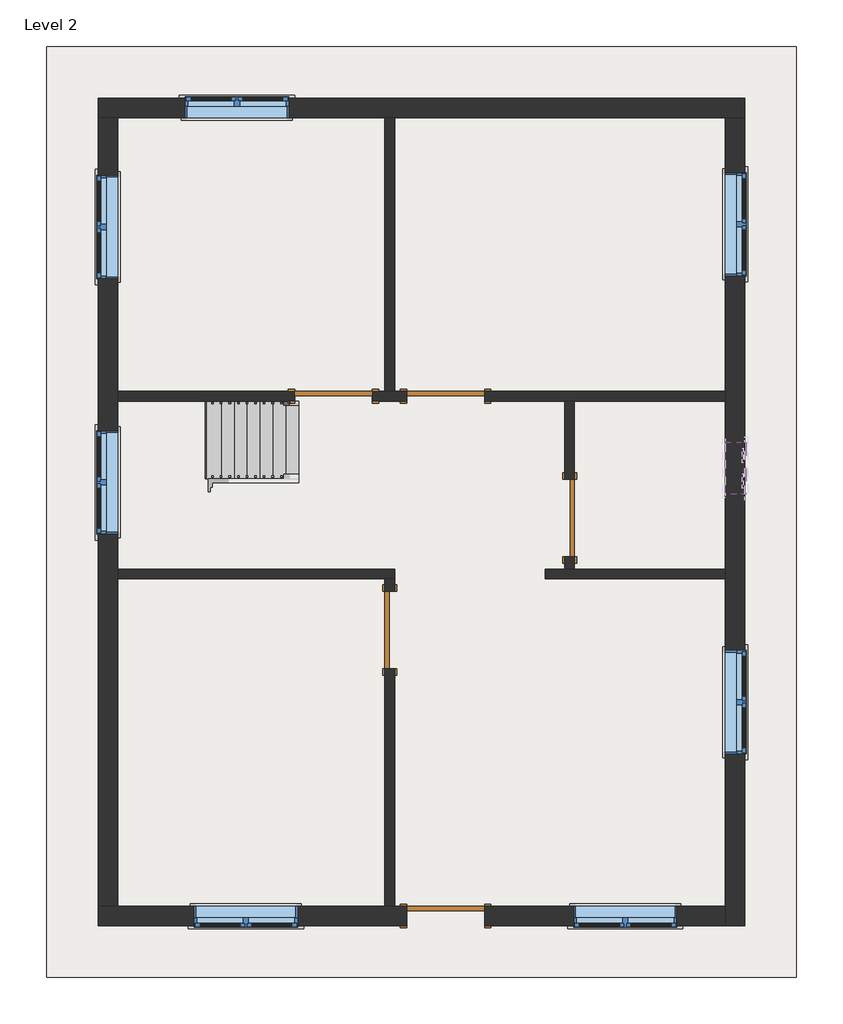
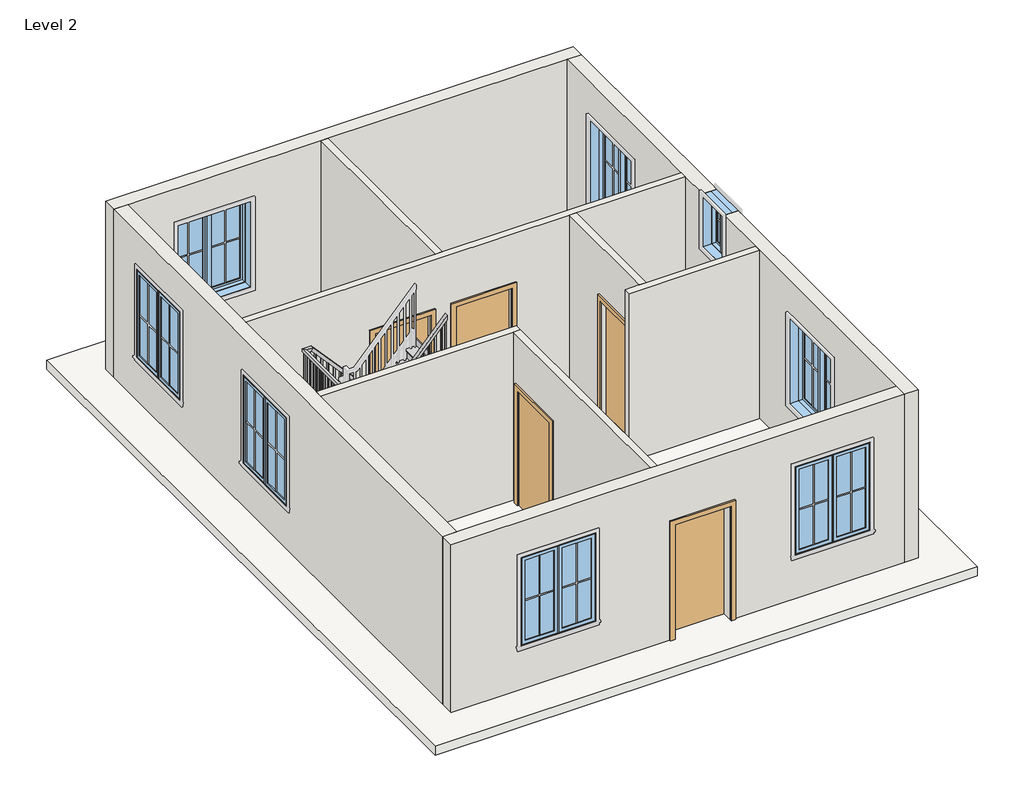
# One storey, part 1 of 2: 10 walls, 8 windows, 5 doors, 1 railing, 1 roof, 1 stair flight.
"""IFC4 building model written with IfcOpenShell, lengths in millimetres."""

from ifc_helpers import new_model, si_unit, frame, origin, place, context, project, spatial, polyline, outline, extrude, faceted_brep, transform, mapped, element, save
from components import door_e5f9f3c4, door_305aa2a5, door_a90ba1ad, stair_flight_8ca9e513, window_c417fced, window_8377141f

model = new_model("IFC4")

# Units and contexts
model_context = context("Model", 3, world=origin())
ifc_project = project(units=[si_unit("LENGTHUNIT", "METRE", prefix="MILLI")], contexts=[model_context])

# Site, building, storey
site = spatial("IfcSite", under=ifc_project)
building = spatial("IfcBuilding", under=site)
storey = spatial("IfcBuildingStorey", under=building, Name="Level 2", Elevation=3048.0)

# Doors
placement = place(None, origin())
door_shape = door_e5f9f3c4(model_context)
element("IfcDoor", 1, ObjectType="Single-Flush : 36\" x 84\"", at=placement, inside=storey, context=model_context, shape_type="MappedRepresentation", body=[
    mapped(door_shape, transform((4044.95, 10966.45, 3048.0), x_axis=(1.0, 0.0, 0.0), y_axis=(0.0, 1.0, 0.0), z_axis=(0.0, 0.0, 1.0))),
])
element("IfcDoor", 2, ObjectType="Single-Flush : 36\" x 84\"", at=placement, inside=storey, context=model_context, shape_type="MappedRepresentation", body=[
    mapped(door_shape, transform((4705.35, 8210.55, 3048.0), x_axis=(0.0, 1.0, 0.0), y_axis=(-1.0, 0.0, 0.0), z_axis=(0.0, 0.0, 1.0))),
])
element("IfcDoor", 3, ObjectType="Single-Flush : 36\" x 84\"", at=placement, inside=storey, context=model_context, shape_type="MappedRepresentation", body=[
    mapped(door_shape, transform((6826.25, 9531.35, 3048.0), x_axis=(0.0, -1.0, 0.0), y_axis=(1.0, 0.0, 0.0), z_axis=(0.0, 0.0, 1.0))),
])
door_2_shape = door_305aa2a5(model_context)
element("IfcDoor", 4, ObjectType="Single-Flush : 36\" x 84\"", at=placement, inside=storey, context=model_context, shape_type="MappedRepresentation", body=[
    mapped(door_2_shape, transform((5365.75, 10966.45, 3048.0), x_axis=(-1.0, 0.0, 0.0), y_axis=(0.0, -1.0, 0.0), z_axis=(0.0, 0.0, 1.0))),
])
door_3_shape = door_a90ba1ad(model_context)
element("IfcDoor", 5, ObjectType="Single-Flush : 36\" x 84\"", at=placement, inside=storey, context=model_context, shape_type="MappedRepresentation", body=[
    mapped(door_3_shape, transform((5365.75, 4838.7, 3048.0), x_axis=(-1.0, 0.0, 0.0), y_axis=(0.0, -1.0, 0.0), z_axis=(0.0, 0.0, 1.0))),
])

# Railing
element("IfcRailing", 6, ObjectType="Handrail - Rectangular", at=placement, inside=storey, context=model_context, shape_type="SolidModel", body=[
    faceted_brep([(3632.2, 10858.5, 4131.7333333), (3632.2, 10858.5, 4055.7950998), (3632.2, 10909.3, 4055.7950998), (3632.2, 10909.3, 4131.7333333), (2565.4, 10858.5, 5317.0666667), (2542.7755898, 10858.5, 5266.2666667), (2542.7755898, 10909.3, 5266.2666667), (2565.4, 10909.3, 5317.0666667), (2463.8, 10858.5, 5317.0666667), (2463.8, 10858.5, 5266.2666667), (2413.0, 10909.3, 5266.2666667), (2413.0, 10909.3, 5317.0666667), (2463.8, 9055.1, 5317.0666667), (2463.8, 9004.3, 5266.2666667), (2413.0, 9004.3, 5266.2666667), (2413.0, 9055.1, 5317.0666667), (2463.8, 9055.1, 5458.1777778), (2463.8, 9004.3, 5407.3777778), (2413.0, 9004.3, 5407.3777778), (2413.0, 9055.1, 5458.1777778), (2463.8, 8978.9, 5458.1777778), (2463.8, 8978.9, 5407.3777778), (2413.0, 8928.1, 5407.3777778), (2413.0, 8928.1, 5458.1777778), (2540.0, 8978.9, 5458.1777778), (2562.6244102, 8978.9, 5407.3777778), (2562.6244102, 8928.1, 5407.3777778), (2540.0, 8928.1, 5458.1777778), (3632.2, 8978.9, 6671.7333333), (3632.2, 8928.1, 6671.7333333), (3632.2, 8928.1, 6595.7950998), (3632.2, 8978.9, 6595.7950998)], [[[0, 1, 2, 3]], [[1, 0, 4, 5]], [[2, 1, 5, 6]], [[3, 2, 6, 7]], [[0, 3, 7, 4]], [[5, 4, 8, 9]], [[6, 5, 9, 10]], [[7, 6, 10, 11]], [[4, 7, 11, 8]], [[9, 8, 12, 13]], [[10, 9, 13, 14]], [[11, 10, 14, 15]], [[8, 11, 15, 12]], [[13, 12, 16, 17]], [[14, 13, 17, 18]], [[15, 14, 18, 19]], [[12, 15, 19, 16]], [[17, 16, 20, 21]], [[18, 17, 21, 22]], [[19, 18, 22, 23]], [[16, 19, 23, 20]], [[21, 20, 24, 25]], [[22, 21, 25, 26]], [[23, 22, 26, 27]], [[20, 23, 27, 24]], [[28, 29, 30, 31]], [[25, 24, 28, 31]], [[26, 25, 31, 30]], [[27, 26, 30, 29]], [[24, 27, 29, 28]]]),
    extrude(outline(polyline([(6521.7117665, 3565.525), (6500.5450998, 3546.475), (5588.0, 3546.475), (5588.0, 3565.525), (6521.7117665, 3565.525)])), frame((0.0, 8943.975, 0.0), z_axis=(0.0, 1.0, 0.0), x_axis=(0.0, 0.0, 1.0)), (0.0, 0.0, 1.0), 19.05),
    extrude(outline(polyline([(6408.8228776, 3463.925), (6387.6562109, 3444.875), (5418.6666667, 3444.875), (5418.6666667, 3463.925), (6408.8228776, 3463.925)])), frame((0.0, 8943.975, 0.0), z_axis=(0.0, 1.0, 0.0), x_axis=(0.0, 0.0, 1.0)), (0.0, 0.0, 1.0), 19.05),
    extrude(outline(polyline([(6295.9339887, 3362.325), (6274.767322, 3343.275), (5418.6666667, 3343.275), (5418.6666667, 3362.325), (6295.9339887, 3362.325)])), frame((0.0, 8943.975, 0.0), z_axis=(0.0, 1.0, 0.0), x_axis=(0.0, 0.0, 1.0)), (0.0, 0.0, 1.0), 19.05),
    extrude(outline(polyline([(6183.0450998, 3260.725), (6161.8784332, 3241.675), (5249.3333333, 3241.675), (5249.3333333, 3260.725), (6183.0450998, 3260.725)])), frame((0.0, 8943.975, 0.0), z_axis=(0.0, 1.0, 0.0), x_axis=(0.0, 0.0, 1.0)), (0.0, 0.0, 1.0), 19.05),
    extrude(outline(polyline([(6070.1562109, 3159.125), (6048.9895443, 3140.075), (5080.0, 3140.075), (5080.0, 3159.125), (6070.1562109, 3159.125)])), frame((0.0, 8943.975, 0.0), z_axis=(0.0, 1.0, 0.0), x_axis=(0.0, 0.0, 1.0)), (0.0, 0.0, 1.0), 19.05),
    extrude(outline(polyline([(5957.267322, 3057.525), (5936.1006554, 3038.475), (5080.0, 3038.475), (5080.0, 3057.525), (5957.267322, 3057.525)])), frame((0.0, 8943.975, 0.0), z_axis=(0.0, 1.0, 0.0), x_axis=(0.0, 0.0, 1.0)), (0.0, 0.0, 1.0), 19.05),
    extrude(outline(polyline([(5844.3784332, 2955.925), (5823.2117665, 2936.875), (4910.6666667, 2936.875), (4910.6666667, 2955.925), (5844.3784332, 2955.925)])), frame((0.0, 8943.975, 0.0), z_axis=(0.0, 1.0, 0.0), x_axis=(0.0, 0.0, 1.0)), (0.0, 0.0, 1.0), 19.05),
    extrude(outline(polyline([(5731.4895443, 2854.325), (5710.3228776, 2835.275), (4741.3333333, 2835.275), (4741.3333333, 2854.325), (5731.4895443, 2854.325)])), frame((0.0, 8943.975, 0.0), z_axis=(0.0, 1.0, 0.0), x_axis=(0.0, 0.0, 1.0)), (0.0, 0.0, 1.0), 19.05),
    extrude(outline(polyline([(5618.6006554, 2752.725), (5597.4339887, 2733.675), (4741.3333333, 2733.675), (4741.3333333, 2752.725), (5618.6006554, 2752.725)])), frame((0.0, 8943.975, 0.0), z_axis=(0.0, 1.0, 0.0), x_axis=(0.0, 0.0, 1.0)), (0.0, 0.0, 1.0), 19.05),
    extrude(outline(polyline([(5505.7117665, 2651.125), (5484.5450998, 2632.075), (4572.0, 2632.075), (4572.0, 2651.125), (5505.7117665, 2651.125)])), frame((0.0, 8943.975, 0.0), z_axis=(0.0, 1.0, 0.0), x_axis=(0.0, 0.0, 1.0)), (0.0, 0.0, 1.0), 19.05),
    extrude(outline(polyline([(5392.8228776, 2549.525), (5371.6562109, 2530.475), (4402.6666667, 2530.475), (4402.6666667, 2549.525), (5392.8228776, 2549.525)])), frame((0.0, 8943.975, 0.0), z_axis=(0.0, 1.0, 0.0), x_axis=(0.0, 0.0, 1.0)), (0.0, 0.0, 1.0), 19.05),
    extrude(outline(polyline([(2428.875, 9064.625), (2447.925, 9064.625), (2447.925, 9045.575), (2428.875, 9045.575), (2428.875, 9064.625)])), frame((0.0, 0.0, 4402.6666667), z_axis=(0.0, 0.0, 1.0), x_axis=(1.0, 0.0, 0.0)), (0.0, 0.0, 1.0), 863.6),
    extrude(outline(polyline([(2428.875, 9166.225), (2447.925, 9166.225), (2447.925, 9147.175), (2428.875, 9147.175), (2428.875, 9166.225)])), frame((0.0, 0.0, 4402.6666667), z_axis=(0.0, 0.0, 1.0), x_axis=(1.0, 0.0, 0.0)), (0.0, 0.0, 1.0), 863.6),
    extrude(outline(polyline([(2428.875, 9267.825), (2447.925, 9267.825), (2447.925, 9248.775), (2428.875, 9248.775), (2428.875, 9267.825)])), frame((0.0, 0.0, 4402.6666667), z_axis=(0.0, 0.0, 1.0), x_axis=(1.0, 0.0, 0.0)), (0.0, 0.0, 1.0), 863.6),
    extrude(outline(polyline([(2428.875, 9369.425), (2447.925, 9369.425), (2447.925, 9350.375), (2428.875, 9350.375), (2428.875, 9369.425)])), frame((0.0, 0.0, 4402.6666667), z_axis=(0.0, 0.0, 1.0), x_axis=(1.0, 0.0, 0.0)), (0.0, 0.0, 1.0), 863.6),
    extrude(outline(polyline([(2428.875, 9471.025), (2447.925, 9471.025), (2447.925, 9451.975), (2428.875, 9451.975), (2428.875, 9471.025)])), frame((0.0, 0.0, 4402.6666667), z_axis=(0.0, 0.0, 1.0), x_axis=(1.0, 0.0, 0.0)), (0.0, 0.0, 1.0), 863.6),
    extrude(outline(polyline([(2428.875, 9572.625), (2447.925, 9572.625), (2447.925, 9553.575), (2428.875, 9553.575), (2428.875, 9572.625)])), frame((0.0, 0.0, 4402.6666667), z_axis=(0.0, 0.0, 1.0), x_axis=(1.0, 0.0, 0.0)), (0.0, 0.0, 1.0), 863.6),
    extrude(outline(polyline([(2428.875, 9674.225), (2447.925, 9674.225), (2447.925, 9655.175), (2428.875, 9655.175), (2428.875, 9674.225)])), frame((0.0, 0.0, 4402.6666667), z_axis=(0.0, 0.0, 1.0), x_axis=(1.0, 0.0, 0.0)), (0.0, 0.0, 1.0), 863.6),
    extrude(outline(polyline([(2428.875, 9775.825), (2447.925, 9775.825), (2447.925, 9756.775), (2428.875, 9756.775), (2428.875, 9775.825)])), frame((0.0, 0.0, 4402.6666667), z_axis=(0.0, 0.0, 1.0), x_axis=(1.0, 0.0, 0.0)), (0.0, 0.0, 1.0), 863.6),
    extrude(outline(polyline([(2428.875, 9877.425), (2447.925, 9877.425), (2447.925, 9858.375), (2428.875, 9858.375), (2428.875, 9877.425)])), frame((0.0, 0.0, 4402.6666667), z_axis=(0.0, 0.0, 1.0), x_axis=(1.0, 0.0, 0.0)), (0.0, 0.0, 1.0), 863.6),
    extrude(outline(polyline([(2428.875, 9979.025), (2447.925, 9979.025), (2447.925, 9959.975), (2428.875, 9959.975), (2428.875, 9979.025)])), frame((0.0, 0.0, 4402.6666667), z_axis=(0.0, 0.0, 1.0), x_axis=(1.0, 0.0, 0.0)), (0.0, 0.0, 1.0), 863.6),
    extrude(outline(polyline([(2428.875, 10080.625), (2447.925, 10080.625), (2447.925, 10061.575), (2428.875, 10061.575), (2428.875, 10080.625)])), frame((0.0, 0.0, 4402.6666667), z_axis=(0.0, 0.0, 1.0), x_axis=(1.0, 0.0, 0.0)), (0.0, 0.0, 1.0), 863.6),
    extrude(outline(polyline([(2428.875, 10182.225), (2447.925, 10182.225), (2447.925, 10163.175), (2428.875, 10163.175), (2428.875, 10182.225)])), frame((0.0, 0.0, 4402.6666667), z_axis=(0.0, 0.0, 1.0), x_axis=(1.0, 0.0, 0.0)), (0.0, 0.0, 1.0), 863.6),
    extrude(outline(polyline([(2428.875, 10283.825), (2447.925, 10283.825), (2447.925, 10264.775), (2428.875, 10264.775), (2428.875, 10283.825)])), frame((0.0, 0.0, 4402.6666667), z_axis=(0.0, 0.0, 1.0), x_axis=(1.0, 0.0, 0.0)), (0.0, 0.0, 1.0), 863.6),
    extrude(outline(polyline([(2428.875, 10385.425), (2447.925, 10385.425), (2447.925, 10366.375), (2428.875, 10366.375), (2428.875, 10385.425)])), frame((0.0, 0.0, 4402.6666667), z_axis=(0.0, 0.0, 1.0), x_axis=(1.0, 0.0, 0.0)), (0.0, 0.0, 1.0), 863.6),
    extrude(outline(polyline([(2428.875, 10487.025), (2447.925, 10487.025), (2447.925, 10467.975), (2428.875, 10467.975), (2428.875, 10487.025)])), frame((0.0, 0.0, 4402.6666667), z_axis=(0.0, 0.0, 1.0), x_axis=(1.0, 0.0, 0.0)), (0.0, 0.0, 1.0), 863.6),
    extrude(outline(polyline([(2428.875, 10588.625), (2447.925, 10588.625), (2447.925, 10569.575), (2428.875, 10569.575), (2428.875, 10588.625)])), frame((0.0, 0.0, 4402.6666667), z_axis=(0.0, 0.0, 1.0), x_axis=(1.0, 0.0, 0.0)), (0.0, 0.0, 1.0), 863.6),
    extrude(outline(polyline([(2428.875, 10690.225), (2447.925, 10690.225), (2447.925, 10671.175), (2428.875, 10671.175), (2428.875, 10690.225)])), frame((0.0, 0.0, 4402.6666667), z_axis=(0.0, 0.0, 1.0), x_axis=(1.0, 0.0, 0.0)), (0.0, 0.0, 1.0), 863.6),
    extrude(outline(polyline([(2428.875, 10791.825), (2447.925, 10791.825), (2447.925, 10772.775), (2428.875, 10772.775), (2428.875, 10791.825)])), frame((0.0, 0.0, 4402.6666667), z_axis=(0.0, 0.0, 1.0), x_axis=(1.0, 0.0, 0.0)), (0.0, 0.0, 1.0), 863.6),
    extrude(outline(polyline([(2524.125, 10893.425), (2524.125, 10874.375), (2505.075, 10874.375), (2505.075, 10893.425), (2524.125, 10893.425)])), frame((0.0, 0.0, 4402.6666667), z_axis=(0.0, 0.0, 1.0), x_axis=(1.0, 0.0, 0.0)), (0.0, 0.0, 1.0), 863.6),
    extrude(outline(polyline([(5174.1006554, 2625.725), (5195.267322, 2606.675), (4233.3333333, 2606.675), (4233.3333333, 2625.725), (5174.1006554, 2625.725)])), frame((0.0, 10874.375, 0.0), z_axis=(0.0, 1.0, 0.0), x_axis=(0.0, 0.0, 1.0)), (0.0, 0.0, 1.0), 19.05),
    extrude(outline(polyline([(5061.2117665, 2727.325), (5082.3784332, 2708.275), (4233.3333333, 2708.275), (4233.3333333, 2727.325), (5061.2117665, 2727.325)])), frame((0.0, 10874.375, 0.0), z_axis=(0.0, 1.0, 0.0), x_axis=(0.0, 0.0, 1.0)), (0.0, 0.0, 1.0), 19.05),
    extrude(outline(polyline([(4948.3228776, 2828.925), (4969.4895443, 2809.875), (4064.0, 2809.875), (4064.0, 2828.925), (4948.3228776, 2828.925)])), frame((0.0, 10874.375, 0.0), z_axis=(0.0, 1.0, 0.0), x_axis=(0.0, 0.0, 1.0)), (0.0, 0.0, 1.0), 19.05),
    extrude(outline(polyline([(4835.4339887, 2930.525), (4856.6006554, 2911.475), (3894.6666667, 2911.475), (3894.6666667, 2930.525), (4835.4339887, 2930.525)])), frame((0.0, 10874.375, 0.0), z_axis=(0.0, 1.0, 0.0), x_axis=(0.0, 0.0, 1.0)), (0.0, 0.0, 1.0), 19.05),
    extrude(outline(polyline([(4722.5450998, 3032.125), (4743.7117665, 3013.075), (3894.6666667, 3013.075), (3894.6666667, 3032.125), (4722.5450998, 3032.125)])), frame((0.0, 10874.375, 0.0), z_axis=(0.0, 1.0, 0.0), x_axis=(0.0, 0.0, 1.0)), (0.0, 0.0, 1.0), 19.05),
    extrude(outline(polyline([(4609.6562109, 3133.725), (4630.8228776, 3114.675), (3725.3333333, 3114.675), (3725.3333333, 3133.725), (4609.6562109, 3133.725)])), frame((0.0, 10874.375, 0.0), z_axis=(0.0, 1.0, 0.0), x_axis=(0.0, 0.0, 1.0)), (0.0, 0.0, 1.0), 19.05),
    extrude(outline(polyline([(4496.767322, 3235.325), (4517.9339887, 3216.275), (3556.0, 3216.275), (3556.0, 3235.325), (4496.767322, 3235.325)])), frame((0.0, 10874.375, 0.0), z_axis=(0.0, 1.0, 0.0), x_axis=(0.0, 0.0, 1.0)), (0.0, 0.0, 1.0), 19.05),
    extrude(outline(polyline([(4383.8784332, 3336.925), (4405.0450998, 3317.875), (3556.0, 3317.875), (3556.0, 3336.925), (4383.8784332, 3336.925)])), frame((0.0, 10874.375, 0.0), z_axis=(0.0, 1.0, 0.0), x_axis=(0.0, 0.0, 1.0)), (0.0, 0.0, 1.0), 19.05),
    extrude(outline(polyline([(4270.9895443, 3438.525), (4292.1562109, 3419.475), (3386.6666667, 3419.475), (3386.6666667, 3438.525), (4270.9895443, 3438.525)])), frame((0.0, 10874.375, 0.0), z_axis=(0.0, 1.0, 0.0), x_axis=(0.0, 0.0, 1.0)), (0.0, 0.0, 1.0), 19.05),
    extrude(outline(polyline([(4158.1006554, 3540.125), (4179.267322, 3521.075), (3217.3333333, 3521.075), (3217.3333333, 3540.125), (4158.1006554, 3540.125)])), frame((0.0, 10874.375, 0.0), z_axis=(0.0, 1.0, 0.0), x_axis=(0.0, 0.0, 1.0)), (0.0, 0.0, 1.0), 19.05),
    extrude(outline(polyline([(2428.875, 8963.025), (2447.925, 8963.025), (2447.925, 8943.975), (2428.875, 8943.975), (2428.875, 8963.025)])), frame((0.0, 0.0, 4402.6666667), z_axis=(0.0, 0.0, 1.0), x_axis=(1.0, 0.0, 0.0)), (0.0, 0.0, 1.0), 1004.7111111),
    extrude(outline(polyline([(2447.925, 10893.425), (2447.925, 10874.375), (2428.875, 10874.375), (2428.875, 10893.425), (2447.925, 10893.425)])), frame((0.0, 0.0, 4402.6666667), z_axis=(0.0, 0.0, 1.0), x_axis=(1.0, 0.0, 0.0)), (0.0, 0.0, 1.0), 863.6),
    extrude(outline(polyline([(6595.7950998, 3632.2), (6574.6284332, 3613.15), (5588.0, 3613.15), (5588.0, 3632.2), (6595.7950998, 3632.2)])), frame((0.0, 8943.975, 0.0), z_axis=(0.0, 1.0, 0.0), x_axis=(0.0, 0.0, 1.0)), (0.0, 0.0, 1.0), 19.05),
    extrude(outline(polyline([(4055.7950998, 3632.2), (4076.9617665, 3613.15), (3217.3333333, 3613.15), (3217.3333333, 3632.2), (4055.7950998, 3632.2)])), frame((0.0, 10874.375, 0.0), z_axis=(0.0, 1.0, 0.0), x_axis=(0.0, 0.0, 1.0)), (0.0, 0.0, 1.0), 19.05),
])

# Roof
element("IfcRoof", 7, ObjectType="Generic - 12\"", at=placement, inside=storey, context=model_context, shape_type="SweptSolid", body=[
    extrude(outline(polyline([(660.4, 15087.6), (9499.6, 15087.6), (9499.6, 4114.8), (660.4, 4114.8), (660.4, 15087.6)])), frame((0.0, 0.0, 3048.0), z_axis=(0.0, 0.0, 1.0), x_axis=(1.0, 0.0, 0.0)), (0.0, 0.0, 1.0), 152.4),
])

# Stair flight
stair_flight_shape = stair_flight_8ca9e513(model_context)
element("IfcStairFlight", 8, ObjectType="2\" Tread 1\" Nosing 1/4\" Riser", at=placement, inside=storey, context=model_context, shape_type="MappedRepresentation", body=[
    mapped(stair_flight_shape, transform((0.0, 0.0, 0.0), x_axis=(1.0, 0.0, 0.0), y_axis=(0.0, 1.0, 0.0), z_axis=(0.0, 0.0, 1.0))),
])

# Walls
element("IfcWall", 9, ObjectType="Generic - 5\"", at=placement, inside=storey, context=model_context, shape_type="SweptSolid", body=[
    extrude(outline(polyline([(4648.2, 11023.6), (4648.2, 14249.4), (4762.5, 14249.4), (4762.5, 11023.6), (4648.2, 11023.6)])), frame((0.0, 0.0, 3048.0), z_axis=(0.0, 0.0, 1.0), x_axis=(1.0, 0.0, 0.0)), (0.0, 0.0, 1.0), 3048.0),
])
element("IfcWall", 10, ObjectType="Generic - 5\"", at=placement, inside=storey, context=model_context, shape_type="Brep", body=[
    faceted_brep([(4502.15, 10909.3, 3048.0), (4908.55, 10909.3, 3048.0), (4908.55, 10909.3, 5181.6), (5822.95, 10909.3, 5181.6), (5822.95, 10909.3, 3048.0), (6769.1, 10909.3, 3048.0), (6883.4, 10909.3, 3048.0), (8661.4, 10909.3, 3048.0), (8661.4, 10909.3, 6096.0), (6883.4, 10909.3, 6096.0), (6769.1, 10909.3, 6096.0), (1498.6, 10909.3, 6096.0), (1498.6, 10909.3, 3048.0), (3587.75, 10909.3, 3048.0), (3587.75, 10909.3, 5181.6), (4502.15, 10909.3, 5181.6), (4908.55, 11023.6, 5181.6), (4908.55, 11023.6, 3048.0), (4762.5, 11023.6, 3048.0), (4648.2, 11023.6, 3048.0), (4502.15, 11023.6, 3048.0), (4502.15, 11023.6, 5181.6), (3587.75, 11023.6, 5181.6), (3587.75, 11023.6, 3048.0), (1498.6, 11023.6, 3048.0), (1498.6, 11023.6, 6096.0), (4648.2, 11023.6, 6096.0), (4762.5, 11023.6, 6096.0), (8661.4, 11023.6, 6096.0), (8661.4, 11023.6, 3048.0), (5822.95, 11023.6, 3048.0), (5822.95, 11023.6, 5181.6)], [[[0, 1, 2, 3, 4, 5, 6, 7, 8, 9, 10, 11, 12, 13, 14, 15]], [[16, 17, 18, 19, 20, 21, 22, 23, 24, 25, 26, 27, 28, 29, 30, 31]], [[13, 12, 24, 23]], [[30, 29, 7, 6, 5, 4]], [[20, 19, 18, 17, 1, 0]], [[11, 10, 9, 8, 28, 27, 26, 25]], [[8, 7, 29, 28]], [[12, 11, 25, 24]], [[21, 20, 0, 15]], [[22, 21, 15, 14]], [[23, 22, 14, 13]], [[2, 1, 17, 16]], [[3, 2, 16, 31]], [[4, 3, 31, 30]]]),
])
element("IfcWall", 11, ObjectType="Generic - 5\"", at=placement, inside=storey, context=model_context, shape_type="SweptSolid", body=[
    extrude(outline(polyline([(9074.15, 5181.6), (9074.15, 3048.0), (8928.1, 3048.0), (8928.1, 6096.0), (10909.3, 6096.0), (10909.3, 3048.0), (9988.55, 3048.0), (9988.55, 5181.6), (9074.15, 5181.6)])), frame((6769.1, 0.0, 0.0), z_axis=(1.0, 0.0, 0.0), x_axis=(0.0, 1.0, 0.0)), (0.0, 0.0, 1.0), 114.3),
])
element("IfcWall", 12, ObjectType="Generic - 5\"", at=placement, inside=storey, context=model_context, shape_type="Brep", body=[
    faceted_brep([(1498.6, 8813.8, 3048.0), (4648.2, 8813.8, 3048.0), (4762.5, 8813.8, 3048.0), (4762.5, 8813.8, 6096.0), (4648.2, 8813.8, 6096.0), (1498.6, 8813.8, 6096.0), (1498.6, 8928.1, 3048.0), (1498.6, 8928.1, 6096.0), (4762.5, 8928.1, 6096.0), (4762.5, 8928.1, 3048.0)], [[[0, 1, 2, 3, 4, 5]], [[6, 7, 8, 9]], [[2, 1, 0, 6, 9]], [[5, 4, 3, 8, 7]], [[0, 5, 7, 6]], [[3, 2, 9, 8]]]),
])
element("IfcWall", 13, ObjectType="Generic - 5\"", at=placement, inside=storey, context=model_context, shape_type="SweptSolid", body=[
    extrude(outline(polyline([(8813.8, 3048.0), (8667.75, 3048.0), (8667.75, 5181.6), (7753.35, 5181.6), (7753.35, 3048.0), (4953.0, 3048.0), (4953.0, 6096.0), (8813.8, 6096.0), (8813.8, 3048.0)])), frame((4648.2, 0.0, 0.0), z_axis=(1.0, 0.0, 0.0), x_axis=(0.0, 1.0, 0.0)), (0.0, 0.0, 1.0), 114.3),
])
element("IfcWall", 14, ObjectType="Generic - 5\"", at=placement, inside=storey, context=model_context, shape_type="Brep", body=[
    faceted_brep([(6540.5050896, 8813.8, 3048.0), (8661.4, 8813.8, 3048.0), (8661.4, 8813.8, 6096.0), (6540.5050896, 8813.8, 6096.0), (6540.5050896, 8928.1, 3048.0), (6540.5050896, 8928.1, 6096.0), (6769.1, 8928.1, 6096.0), (6883.4, 8928.1, 6096.0), (8661.4, 8928.1, 6096.0), (8661.4, 8928.1, 3048.0), (6883.4, 8928.1, 3048.0), (6769.1, 8928.1, 3048.0)], [[[0, 1, 2, 3]], [[4, 5, 6, 7, 8, 9, 10, 11]], [[1, 0, 4, 11, 10, 9]], [[3, 2, 8, 7, 6, 5]], [[0, 3, 5, 4]], [[2, 1, 9, 8]]]),
])
element("IfcWall", 15, ObjectType="Generic - 8\"", at=placement, inside=storey, context=model_context, shape_type="Brep", body=[
    faceted_brep([(1270.0, 14249.4, 3048.0), (1498.6, 14249.4, 3048.0), (4648.2, 14249.4, 3048.0), (4762.5, 14249.4, 3048.0), (8661.4, 14249.4, 3048.0), (8890.0, 14249.4, 3048.0), (8890.0, 14249.4, 6096.0), (8661.4, 14249.4, 6096.0), (4762.5, 14249.4, 6096.0), (4648.2, 14249.4, 6096.0), (1498.6, 14249.4, 6096.0), (1270.0, 14249.4, 6096.0), (3514.725, 14249.4, 5486.4), (3514.725, 14249.4, 3962.4), (2295.525, 14249.4, 3962.4), (2295.525, 14249.4, 5486.4), (1270.0, 14478.0, 3048.0), (1270.0, 14478.0, 6096.0), (8890.0, 14478.0, 6096.0), (8890.0, 14478.0, 3048.0), (3514.725, 14478.0, 5486.4), (2295.525, 14478.0, 5486.4), (2295.525, 14478.0, 3962.4), (3514.725, 14478.0, 3962.4)], [[[0, 1, 2, 3, 4, 5, 6, 7, 8, 9, 10, 11], [12, 13, 14, 15]], [[16, 17, 18, 19], [20, 21, 22, 23]], [[5, 4, 3, 2, 1, 0, 16, 19]], [[11, 10, 9, 8, 7, 6, 18, 17]], [[6, 5, 19, 18]], [[0, 11, 17, 16]], [[13, 12, 20, 23]], [[14, 13, 23, 22]], [[15, 14, 22, 21]], [[12, 15, 21, 20]]]),
])
element("IfcWall", 16, ObjectType="Generic - 8\"", at=placement, inside=storey, context=model_context, shape_type="Brep", body=[
    faceted_brep([(8661.4, 14249.4, 3048.0), (8661.4, 11023.6, 3048.0), (8661.4, 10909.3, 3048.0), (8661.4, 8928.1, 3048.0), (8661.4, 8813.8, 3048.0), (8661.4, 4953.0, 3048.0), (8661.4, 4724.4, 3048.0), (8661.4, 4724.4, 6096.0), (8661.4, 4953.0, 6096.0), (8661.4, 8813.8, 6096.0), (8661.4, 8928.1, 6096.0), (8661.4, 9810.75, 6096.0), (8661.4, 9810.75, 5181.6), (8661.4, 10420.35, 5181.6), (8661.4, 10420.35, 6096.0), (8661.4, 10909.3, 6096.0), (8661.4, 11023.6, 6096.0), (8661.4, 14249.4, 6096.0), (8661.4, 6750.05, 5486.4), (8661.4, 6750.05, 3962.4), (8661.4, 7969.25, 3962.4), (8661.4, 7969.25, 5486.4), (8661.4, 12382.5, 5486.4), (8661.4, 12382.5, 3962.4), (8661.4, 13601.7, 3962.4), (8661.4, 13601.7, 5486.4), (8890.0, 4724.4, 3048.0), (8890.0, 14249.4, 3048.0), (8890.0, 14249.4, 6096.0), (8890.0, 10420.35, 6096.0), (8890.0, 10420.35, 5181.6), (8890.0, 9810.75, 5181.6), (8890.0, 9810.75, 6096.0), (8890.0, 4724.4, 6096.0), (8890.0, 6750.05, 3962.4), (8890.0, 6750.05, 5486.4), (8890.0, 7969.25, 5486.4), (8890.0, 7969.25, 3962.4), (8890.0, 12382.5, 3962.4), (8890.0, 12382.5, 5486.4), (8890.0, 13601.7, 5486.4), (8890.0, 13601.7, 3962.4)], [[[0, 1, 2, 3, 4, 5, 6, 7, 8, 9, 10, 11, 12, 13, 14, 15, 16, 17], [18, 19, 20, 21], [22, 23, 24, 25]], [[26, 27, 28, 29, 30, 31, 32, 33], [34, 35, 36, 37], [38, 39, 40, 41]], [[6, 5, 4, 3, 2, 1, 0, 27, 26]], [[28, 17, 16, 15, 14, 29]], [[7, 33, 32, 11, 10, 9, 8]], [[0, 17, 28, 27]], [[7, 6, 26, 33]], [[19, 18, 35, 34]], [[20, 19, 34, 37]], [[21, 20, 37, 36]], [[18, 21, 36, 35]], [[23, 22, 39, 38]], [[24, 23, 38, 41]], [[25, 24, 41, 40]], [[22, 25, 40, 39]], [[31, 12, 11, 32]], [[12, 31, 30, 13]], [[13, 30, 29, 14]]]),
])
element("IfcWall", 17, ObjectType="Generic - 8\"", at=placement, inside=storey, context=model_context, shape_type="Brep", body=[
    faceted_brep([(4908.55, 4953.0, 5181.6), (4908.55, 4953.0, 3048.0), (4762.5, 4953.0, 3048.0), (4648.2, 4953.0, 3048.0), (1498.6, 4953.0, 3048.0), (1270.0, 4953.0, 3048.0), (1270.0, 4953.0, 6096.0), (1498.6, 4953.0, 6096.0), (4648.2, 4953.0, 6096.0), (4762.5, 4953.0, 6096.0), (8661.4, 4953.0, 6096.0), (8661.4, 4953.0, 3048.0), (5822.95, 4953.0, 3048.0), (5822.95, 4953.0, 5181.6), (2400.3, 4953.0, 5486.4), (2400.3, 4953.0, 3962.4), (3619.5, 4953.0, 3962.4), (3619.5, 4953.0, 5486.4), (6872.2875, 4953.0, 5486.4), (6872.2875, 4953.0, 3962.4), (8091.4875, 4953.0, 3962.4), (8091.4875, 4953.0, 5486.4), (1270.0, 4724.4, 3048.0), (4908.55, 4724.4, 3048.0), (4908.55, 4724.4, 5181.6), (5822.95, 4724.4, 5181.6), (5822.95, 4724.4, 3048.0), (8661.4, 4724.4, 3048.0), (8661.4, 4724.4, 6096.0), (1270.0, 4724.4, 6096.0), (2400.3, 4724.4, 5486.4), (3619.5, 4724.4, 5486.4), (3619.5, 4724.4, 3962.4), (2400.3, 4724.4, 3962.4), (6872.2875, 4724.4, 5486.4), (8091.4875, 4724.4, 5486.4), (8091.4875, 4724.4, 3962.4), (6872.2875, 4724.4, 3962.4)], [[[0, 1, 2, 3, 4, 5, 6, 7, 8, 9, 10, 11, 12, 13], [14, 15, 16, 17], [18, 19, 20, 21]], [[22, 23, 24, 25, 26, 27, 28, 29], [30, 31, 32, 33], [34, 35, 36, 37]], [[12, 11, 27, 26]], [[5, 4, 3, 2, 1, 23, 22]], [[10, 9, 8, 7, 6, 29, 28]], [[11, 10, 28, 27]], [[6, 5, 22, 29]], [[24, 23, 1, 0]], [[25, 24, 0, 13]], [[26, 25, 13, 12]], [[15, 14, 30, 33]], [[16, 15, 33, 32]], [[17, 16, 32, 31]], [[14, 17, 31, 30]], [[19, 18, 34, 37]], [[20, 19, 37, 36]], [[21, 20, 36, 35]], [[18, 21, 35, 34]]]),
])
element("IfcWall", 18, ObjectType="Generic - 8\"", at=placement, inside=storey, context=model_context, shape_type="Brep", body=[
    faceted_brep([(1498.6, 4953.0, 3048.0), (1498.6, 8813.8, 3048.0), (1498.6, 8928.1, 3048.0), (1498.6, 10909.3, 3048.0), (1498.6, 11023.6, 3048.0), (1498.6, 14249.4, 3048.0), (1498.6, 14249.4, 6096.0), (1498.6, 11023.6, 6096.0), (1498.6, 10909.3, 6096.0), (1498.6, 8928.1, 6096.0), (1498.6, 8813.8, 6096.0), (1498.6, 4953.0, 6096.0), (1498.6, 13569.95, 5486.4), (1498.6, 13569.95, 3962.4), (1498.6, 12350.75, 3962.4), (1498.6, 12350.75, 5486.4), (1498.6, 10560.05, 5486.4), (1498.6, 10560.05, 3962.4), (1498.6, 9340.85, 3962.4), (1498.6, 9340.85, 5486.4), (1270.0, 14249.4, 3048.0), (1270.0, 4953.0, 3048.0), (1270.0, 4953.0, 6096.0), (1270.0, 14249.4, 6096.0), (1270.0, 13569.95, 3962.4), (1270.0, 13569.95, 5486.4), (1270.0, 12350.75, 5486.4), (1270.0, 12350.75, 3962.4), (1270.0, 10560.05, 3962.4), (1270.0, 10560.05, 5486.4), (1270.0, 9340.85, 5486.4), (1270.0, 9340.85, 3962.4)], [[[0, 1, 2, 3, 4, 5, 6, 7, 8, 9, 10, 11], [12, 13, 14, 15], [16, 17, 18, 19]], [[20, 21, 22, 23], [24, 25, 26, 27], [28, 29, 30, 31]], [[5, 4, 3, 2, 1, 0, 21, 20]], [[11, 10, 9, 8, 7, 6, 23, 22]], [[6, 5, 20, 23]], [[0, 11, 22, 21]], [[13, 12, 25, 24]], [[14, 13, 24, 27]], [[15, 14, 27, 26]], [[12, 15, 26, 25]], [[17, 16, 29, 28]], [[18, 17, 28, 31]], [[19, 18, 31, 30]], [[16, 19, 30, 29]]]),
])

# Windows
window_shape = window_c417fced(model_context)
element("IfcWindow", 19, ObjectType="Window-Casement-Double : 24\" x 36\"", at=placement, inside=storey, context=model_context, shape_type="MappedRepresentation", body=[
    mapped(window_shape, transform((8775.7, 10115.55, 4267.2), x_axis=(0.0, -1.0, 0.0), y_axis=(1.0, 0.0, 0.0), z_axis=(0.0, 0.0, 1.0))),
])
window_2_shape = window_8377141f(model_context)
element("IfcWindow", 20, ObjectType="Window-Casement-Double : 48\" x 60\"", at=placement, inside=storey, context=model_context, shape_type="MappedRepresentation", body=[
    mapped(window_2_shape, transform((7481.8875, 4838.7, 3048.0), x_axis=(-1.0, 0.0, 0.0), y_axis=(0.0, -1.0, 0.0), z_axis=(0.0, 0.0, 1.0))),
])
element("IfcWindow", 21, ObjectType="Window-Casement-Double : 48\" x 60\"", at=placement, inside=storey, context=model_context, shape_type="MappedRepresentation", body=[
    mapped(window_2_shape, transform((3009.9, 4838.7, 3048.0), x_axis=(-1.0, 0.0, 0.0), y_axis=(0.0, -1.0, 0.0), z_axis=(0.0, 0.0, 1.0))),
])
element("IfcWindow", 22, ObjectType="Window-Casement-Double : 48\" x 60\"", at=placement, inside=storey, context=model_context, shape_type="MappedRepresentation", body=[
    mapped(window_2_shape, transform((8775.7, 12992.1, 3048.0), x_axis=(0.0, -1.0, 0.0), y_axis=(1.0, 0.0, 0.0), z_axis=(0.0, 0.0, 1.0))),
])
element("IfcWindow", 23, ObjectType="Window-Casement-Double : 48\" x 60\"", at=placement, inside=storey, context=model_context, shape_type="MappedRepresentation", body=[
    mapped(window_2_shape, transform((8775.7, 7359.65, 3048.0), x_axis=(0.0, -1.0, 0.0), y_axis=(1.0, 0.0, 0.0), z_axis=(0.0, 0.0, 1.0))),
])
element("IfcWindow", 24, ObjectType="Window-Casement-Double : 48\" x 60\"", at=placement, inside=storey, context=model_context, shape_type="MappedRepresentation", body=[
    mapped(window_2_shape, transform((1384.3, 12960.35, 3048.0), x_axis=(0.0, 1.0, 0.0), y_axis=(-1.0, 0.0, 0.0), z_axis=(0.0, 0.0, 1.0))),
])
element("IfcWindow", 25, ObjectType="Window-Casement-Double : 48\" x 60\"", at=placement, inside=storey, context=model_context, shape_type="MappedRepresentation", body=[
    mapped(window_2_shape, transform((1384.3, 9950.45, 3048.0), x_axis=(0.0, 1.0, 0.0), y_axis=(-1.0, 0.0, 0.0), z_axis=(0.0, 0.0, 1.0))),
])
element("IfcWindow", 26, ObjectType="Window-Casement-Double : 48\" x 60\"", at=placement, inside=storey, context=model_context, shape_type="MappedRepresentation", body=[
    mapped(window_2_shape, transform((2905.125, 14363.7, 3048.0), x_axis=(1.0, 0.0, 0.0), y_axis=(0.0, 1.0, 0.0), z_axis=(0.0, 0.0, 1.0))),
])

save(model, "model.ifc")

# Revit data of these elements
# Type "Single-Flush : 36\" x 84\""
#   Type Mark = "1"
#   Construction Type Id = "MDOOR"
#   Assembly Code = "C1020"
#   Analytic Construction = "Metal"
#   Thickness = 0' - 2"
#   Heat Transfer Coefficient (U) = 0.651978 BTU/(h·ft²·°F)
#   Height = 7' - 0"
#   Trim Projection Ext = 0' - 1"
#   Trim Projection Int = 0' - 1"
#   Trim Width = 0' - 3"
#   Width = 3' - 0"
#   Define Thermal Properties by = 1
#   Define Thermal Properties by = 1
#   Door Material = Door - Panel
#   Frame Material = Door - Frame
#   Visual Light Transmittance = 0
#   Solar Heat Gain Coefficient = 0
#   Function = (empty or 0)
#   Wall Closure = (empty or 0)
# Type "Handrail - Rectangular"
#   Assembly Code = "C2010400"
#   built-in parameter 1008612 = 0.0416667 (stored number, unit not read)
#   built-in parameter 1008611 = 0.0416667 (stored number, unit not read)
#   built-in parameter 1008609 = 0.333333 (stored number, unit not read)
#   built-in parameter 1008604 = 0.166667 (stored number, unit not read)
#   built-in parameter 1008603 = 0.166667 (stored number, unit not read)
#   Railing Height = 3' - 0"
#   built-in parameter 1008630 = 2
#   built-in parameter 1008610 = 2
#   built-in parameter 1008618 = Baluster - Square : 3/4"
# Type "Generic - 12\""
#   Assembly Code = "B1020"
#   Layers, outside or top first: 0' - 6" no material (function 1)
# Type "Generic - 5\""
#   Assembly Code = "B2010"
#   Layers, outside or top first: 0' - 4 1/2" no material (function 1)
# Type "Generic - 8\""
#   Assembly Code = "B2010"
#   Layers, outside or top first: 0' - 9" "Parking Stripe" (function 1)
# Type "Window-Casement-Double : 24\" x 36\""
#   Type Mark = "14"
#   Fire Rating = "0.5h"
#   Assembly Code = "B2020100"
#   Analytic Construction = "Double glazing - domestic"
#   Frame Extension [instance default] = 0' - 0 1/4"
#   Window Inset [instance default] = 0' - 0"
#   Wall Thickness [instance default] = 0' - 6"
#   Interior Wall Closure [instance default] = 0' - 2 1/4"
#   Half Width = 1' - 0"
#   Visual Light Transmittance = 0.81
#   Thermal Resistance (R) = 1.8146 (h·ft²·°F)/BTU
#   Solar Heat Gain Coefficient = 0.76
#   Rough Width = 2' - 0 1/2"
#   Rough Height = 3' - 0 1/2"
#   Height = 3' - 0"
#   Heat Transfer Coefficient (U) = 0.5511 BTU/(h·ft²·°F)
#   Exterior Wall Closure [instance default] = 0' - 1 1/4"
#   Extension Jamb [instance default] = 0' - 2 1/4"
#   Default Sill Height = 3' - 0"
#   Width = 2' - 0"
#   Define Thermal Properties by = 0
#   Muntin Visibility = yes
#   Interior Trim Visibility [instance default] = yes
#   Exterior Trim Visibility [instance default] = yes
#   Extension Jamb Visibility [instance default] = yes
#   Interior Trim Material = Wood - Stained
#   Muntin Pattern = Muntin Pattern_2x2 : Muntin Pattern_2x2
#   Interior Trim = Trim-Window-Interior-Flat : Picture Frame
#   Interior Frame Material = Wood - Stained
#   Glass Panel Material = Glass
#   Exterior Trim Material = Clad - White
#   Exterior Trim = Trim-Window-Exterior-Flat : with Sill
#   Exterior Frame Material = Clad - White
#   Wall Closure = (empty or 0)
# Type "Window-Casement-Double : 48\" x 60\""
#   Type Mark = "17"
#   Fire Rating = "0.5h"
#   Assembly Code = "B2020100"
#   Analytic Construction = "Double glazing - domestic"
#   Frame Extension [instance default] = 0' - 0 1/4"
#   Window Inset [instance default] = 0' - 0"
#   Wall Thickness [instance default] = 0' - 6"
#   Interior Wall Closure [instance default] = 0' - 2 1/4"
#   Half Width = 2' - 0"
#   Visual Light Transmittance = 0.81
#   Thermal Resistance (R) = 1.8146 (h·ft²·°F)/BTU
#   Solar Heat Gain Coefficient = 0.76
#   Rough Width = 4' - 0 1/2"
#   Rough Height = 5' - 0 1/2"
#   Height = 5' - 0"
#   Heat Transfer Coefficient (U) = 0.5511 BTU/(h·ft²·°F)
#   Exterior Wall Closure [instance default] = 0' - 1 1/4"
#   Extension Jamb [instance default] = 0' - 2 1/4"
#   Default Sill Height = 3' - 0"
#   Width = 4' - 0"
#   Define Thermal Properties by = 0
#   Muntin Visibility = yes
#   Interior Trim Visibility [instance default] = yes
#   Exterior Trim Visibility [instance default] = yes
#   Extension Jamb Visibility [instance default] = yes
#   Interior Trim Material = Wood - Stained
#   Muntin Pattern = Muntin Pattern_2x2 : Muntin Pattern_2x2
#   Interior Trim = Trim-Window-Interior-Flat : Picture Frame
#   Interior Frame Material = Wood - Stained
#   Glass Panel Material = Glass
#   Exterior Trim Material = Clad - White
#   Exterior Trim = Trim-Window-Exterior-Flat : with Sill
#   Exterior Frame Material = Clad - White
#   Wall Closure = (empty or 0)
# Elements 1, 2, 3, 4, 5 (IfcDoor, "Single-Flush : 36\" x 84\"")
#   Phase Created = New Construction
#   Materials on its faces: "Door - Frame", "Door - Panel"
# Element 6 (IfcRailing, "Handrail - Rectangular")
#   Phase Created = New Construction
# Element 7 (IfcRoof, "Generic - 12\"")
#   built-in parameter 1001705 = 10.5 (stored number, unit not read)
#   built-in parameter 1001710 = 33615
#   Phase Created = New Construction
#   Materials on its faces: "Textile - Linen, Smooth", "Default Roof"
# Element 8 (IfcStairFlight, "2\" Tread 1\" Nosing 1/4\" Riser")
#   Phase Created = New Construction
# Elements 9, 10, 11, 12, 13, 14 (IfcWall, "Generic - 5\"")
#   Top Offset = 0' - 0"
#   Base Offset = 0' - 0"
#   wall height = 10' - 0"
#   Phase Created = New Construction
#   Base Constraint = Level 2
#   Top Constraint = Level 3
#   Materials on its faces: "Default Wall"
# Elements 15, 16, 17, 18 (IfcWall, "Generic - 8\"")
#   Top Offset = 0' - 0"
#   Base Offset = 0' - 0"
#   Unconnected Height = 10' - 0"
#   wall height = 10' - 0"
#   Phase Created = New Construction
#   Base Constraint = Level 2
#   Materials on its faces: "Parking Stripe", "Wood Planks"
# Element 19 (IfcWindow, "Window-Casement-Double : 24\" x 36\"")
#   Mark = "21"
#   Window Inset = 0' - 0"
#   Interior Wall Closure = 0' - 2 1/4"
#   Frame Extension = 0' - 0 1/4"
#   Exterior Wall Closure = 0' - 1 1/4"
#   Interior Trim Visibility = yes
#   Exterior Trim Visibility = yes
#   Phase Created = New Construction
#   Materials on its faces: "Wood - Stained", "Glass", "Clad - White"
# Element 20 (IfcWindow, "Window-Casement-Double : 48\" x 60\"")
#   Mark = "9"
#   Window Inset = 0' - 0"
#   Interior Wall Closure = 0' - 2 1/4"
#   Frame Extension = 0' - 0 1/4"
#   Exterior Wall Closure = 0' - 1 1/4"
#   Interior Trim Visibility = yes
#   Exterior Trim Visibility = yes
#   Phase Created = New Construction
#   Materials on its faces: "Wood - Stained", "Glass", "Clad - White"
# Element 21 (IfcWindow, "Window-Casement-Double : 48\" x 60\"")
#   Mark = "10"
#   Window Inset = 0' - 0"
#   Interior Wall Closure = 0' - 2 1/4"
#   Frame Extension = 0' - 0 1/4"
#   Exterior Wall Closure = 0' - 1 1/4"
#   Interior Trim Visibility = yes
#   Exterior Trim Visibility = yes
#   Phase Created = New Construction
#   Materials on its faces: "Wood - Stained", "Glass", "Clad - White"
# Element 22 (IfcWindow, "Window-Casement-Double : 48\" x 60\"")
#   Mark = "19"
#   Window Inset = 0' - 0"
#   Interior Wall Closure = 0' - 2 1/4"
#   Frame Extension = 0' - 0 1/4"
#   Exterior Wall Closure = 0' - 1 1/4"
#   Interior Trim Visibility = yes
#   Exterior Trim Visibility = yes
#   Phase Created = New Construction
#   Materials on its faces: "Wood - Stained", "Glass", "Clad - White"
# Element 23 (IfcWindow, "Window-Casement-Double : 48\" x 60\"")
#   Mark = "20"
#   Window Inset = 0' - 0"
#   Interior Wall Closure = 0' - 2 1/4"
#   Frame Extension = 0' - 0 1/4"
#   Exterior Wall Closure = 0' - 1 1/4"
#   Interior Trim Visibility = yes
#   Exterior Trim Visibility = yes
#   Phase Created = New Construction
#   Materials on its faces: "Wood - Stained", "Glass", "Clad - White"
# Element 24 (IfcWindow, "Window-Casement-Double : 48\" x 60\"")
#   Mark = "34"
#   Window Inset = 0' - 0"
#   Interior Wall Closure = 0' - 2 1/4"
#   Frame Extension = 0' - 0 1/4"
#   Exterior Wall Closure = 0' - 1 1/4"
#   Interior Trim Visibility = yes
#   Exterior Trim Visibility = yes
#   Phase Created = New Construction
#   Materials on its faces: "Wood - Stained", "Glass", "Clad - White"
# Element 25 (IfcWindow, "Window-Casement-Double : 48\" x 60\"")
#   Mark = "38"
#   Window Inset = 0' - 0"
#   Interior Wall Closure = 0' - 2 1/4"
#   Frame Extension = 0' - 0 1/4"
#   Exterior Wall Closure = 0' - 1 1/4"
#   Interior Trim Visibility = yes
#   Exterior Trim Visibility = yes
#   Phase Created = New Construction
#   Materials on its faces: "Wood - Stained", "Glass", "Clad - White"
# Element 26 (IfcWindow, "Window-Casement-Double : 48\" x 60\"")
#   Mark = "48"
#   Window Inset = 0' - 0"
#   Interior Wall Closure = 0' - 2 1/4"
#   Frame Extension = 0' - 0 1/4"
#   Exterior Wall Closure = 0' - 1 1/4"
#   Interior Trim Visibility = yes
#   Exterior Trim Visibility = yes
#   Phase Created = New Construction
#   Materials on its faces: "Wood - Stained", "Glass", "Clad - White"
# Materials
#   "Door - Panel": class "Wood", colour RGB 210 159 95, transparency 0, Cost = 0
#   "Door - Frame": colour RGB 118 70 51, transparency 0, Cost = 0
#   "Parking Stripe": class "Paint", colour RGB 250 250 91, transparency 0, Cost = 0
#   "Wood - Stained": class "Wood", colour RGB 224 178 126, transparency 0, Cost = 0
#   "Glass": class "Glass", colour RGB 0 128 192, transparency 0.75, Description = "Soda Lime Glass", Cost = 0
#   "Clad - White": class "Wood", colour RGB 242 242 238, transparency 0, Cost = 0
#   "Textile - Linen, Smooth": colour RGB 249 239 230, transparency 0
#   "Default Roof": colour RGB 88 101 114, transparency 0, Cost = 0
#   "Default Wall": colour RGB 128 128 128, transparency 0, Cost = 0
#   "Wood Planks": class "Wood", colour RGB 193 160 115, transparency 0, Description = "Physical material.", Cost = 0
